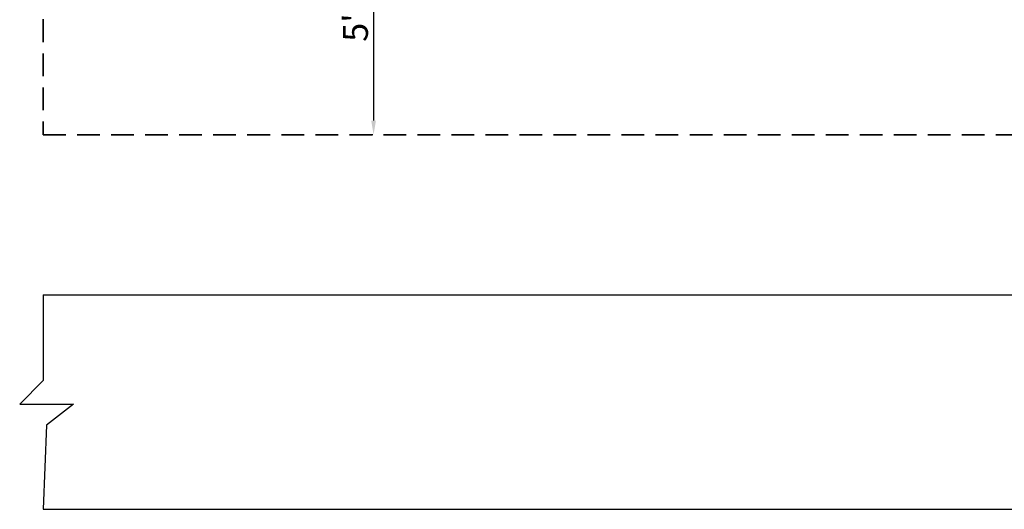
# Model space of a CAD drawing. Units: inches. Extents: x -7 to 1228, y -146 to 1091.
# Tile 1 of 88: x -7 to 269, y -105 to 32. Entities that reach past the tile are written whole.
import ezdxf

# ---------------------------------------------------------------- set-up
doc = ezdxf.new("R2010")
doc.units = ezdxf.units.IN
doc.linetypes.add('DASHED2', pattern=[9.525, 6.35, -3.175])
for name, color, linetype, lineweight in [('A-ANNO-DIMS', 2, 'Continuous', 18), ('C-PROP', 1, 'DASHED2', 35), ('C-ROAD', 7, 'Continuous', 25)]:
    doc.layers.add(name, color=color, linetype=linetype, lineweight=lineweight)
doc.styles.get("Standard").update_dxf_attribs({"font": 'arial.ttf'})
doc.dimstyles.new('ISO-25', dxfattribs={"dimtxt": 7, "dimasz": 4, "dimexe": 1.25, "dimexo": 0.625, "dimtad": 1, "dimdec": 1, "dimlunit": 3, "dimtxsty": 'Standard', "dimcen": 2.5, "dimadec": 0, "dimazin": 0, "dimtfac": 1, "dimtdec": 1, "dimtmove": 1, "dimatfit": 3, "dimfxl": 1, "dimarcsym": 0})

# ---------------------------------------------------------------- blocks, each defined once
blk = doc.blocks.new('*D9')
at = {"layer": 'A-ANNO-DIMS', "color": 0, "lineweight": -2, "transparency": 16777216}
for p, q in [((92.31, 60), (91.25, 60)), ((92.5, 56), (92.5, 4)), ((92.31, 0), (91.25, 0))]:
    blk.add_line(p, q, dxfattribs=at)
at = {"layer": 'A-ANNO-DIMS', "color": 0, "transparency": 16777216}
for points in [[(91.83, 56), (93.16, 56), (92.5, 60)], [(91.83, 4), (93.16, 4), (92.5, 0)]]:
    blk.add_solid(points, dxfattribs=at)
at = {"layer": 'Defpoints', "color": 0, "transparency": 16777216}
for p in [(92.94, 60), (92.94, 0), (92.5, 0)]:
    blk.add_point(p, dxfattribs=at)
at = {"layer": 'A-ANNO-DIMS', "color": 0, "transparency": 16777216, "insert": (88.31, 30), "char_height": 7, "attachment_point": 5, "rotation": 90}
blk.add_mtext("5'", dxfattribs=at)

msp = doc.modelspace()

# ---------------------------------------------------------------- linework, layer by layer
at = {"layer": 'C-PROP'}
for p, q in [((0, 1061), (0, 0)), ((0, 0), (1187, 0))]:
    msp.add_line(p, q, dxfattribs=at)
at = {"layer": 'C-ROAD'}
for p, q in [((0, -44.69), (1187, -44.69)), ((0, -44.69), (0, -68.64)), ((0, -68.64), (-6.57, -75.3)), ((-6.57, -75.3), (8.46, -75.3)), ((8.46, -75.3), (0.95, -81.15)), ((0.95, -81.15), (0, -104.69)), ((0, -104.69), (1187, -104.69))]:
    msp.add_line(p, q, dxfattribs=at)

# ---------------------------------------------------------------- dimensions: what is measured, and where the dimension line sits
at = {"layer": 'A-ANNO-DIMS'}
dim = msp.add_linear_dim(base=(92.5, 0), p1=(92.94, 60), p2=(92.94, 0), angle=90, dimstyle='ISO-25', override={"dimclrd": 0, "dimclre": 0, "dimclrt": 0}, dxfattribs=at)
dim.commit()
dim.dimension.update_dxf_attribs({"geometry": '*D9', "text_midpoint": (88.31, 30)})

doc.saveas('drawing.dxf')
